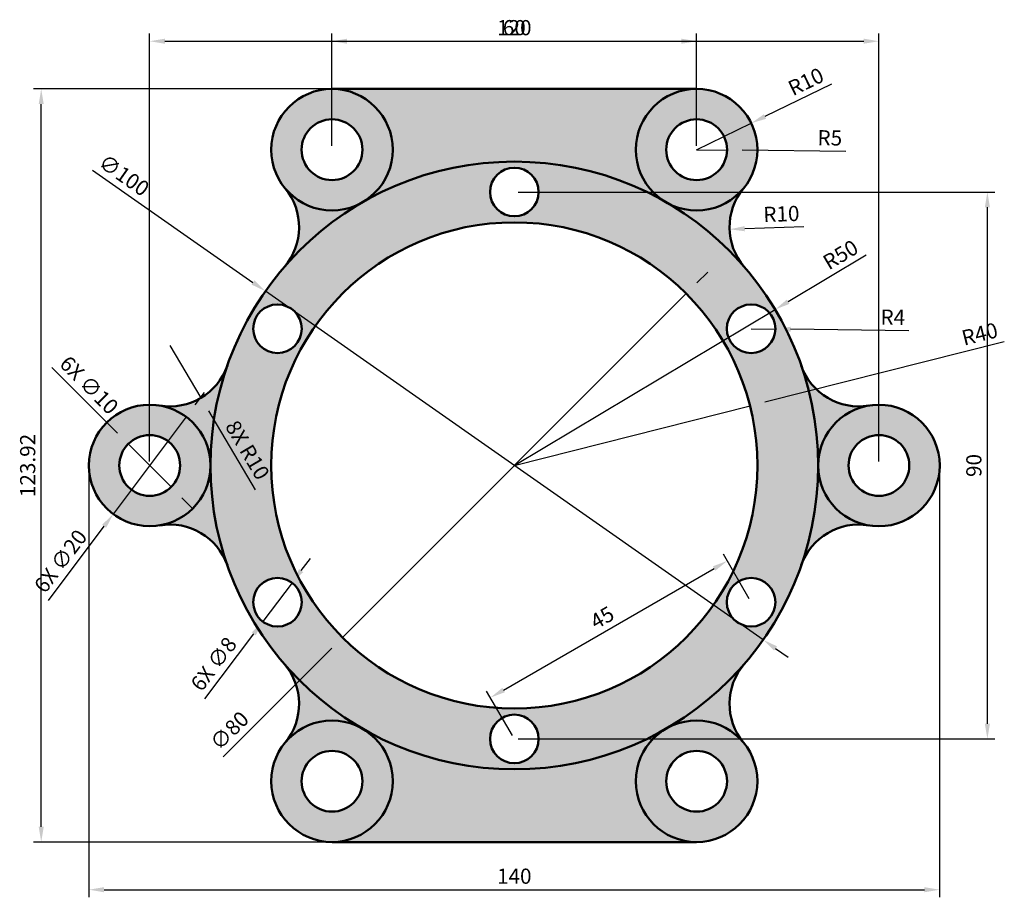
# Model space of a CAD drawing. Units: millimetres. Extents: x 1930 to 2092, y 1732 to 1877.
import ezdxf

# ---------------------------------------------------------------- set-up
doc = ezdxf.new("R2010")
doc.units = ezdxf.units.MM
for name, color, linetype, lineweight in [('M-DIMS', 2, 'Continuous', 25), ('M-HATC', 8, 'Continuous', 18), ('M-OUTL', 7, 'Continuous', 50)]:
    doc.layers.add(name, color=color, linetype=linetype, lineweight=lineweight)
doc.styles.get("Standard").update_dxf_attribs({"font": 'arial.ttf'})
doc.dimstyles.new('ISO-25', dxfattribs={"dimtxt": 2.5, "dimasz": 2.5, "dimexe": 1.25, "dimexo": 0.625, "dimtad": 1, "dimtxsty": 'Standard', "dimcen": 2.5, "dimadec": 0, "dimazin": 0, "dimtfac": 1, "dimtmove": 0, "dimatfit": 3, "dimfxl": 1, "dimarcsym": 0})

# ---------------------------------------------------------------- blocks, each defined once
blk = doc.blocks.new('*D1')
at = {"layer": 'Defpoints', "color": 0, "transparency": 16777216}
for p in [(2050.52, 1859.84), (2041.52, 1855.47)]:
    blk.add_point(p, dxfattribs=at)
at = {"layer": 'M-DIMS', "color": 0, "lineweight": -2, "transparency": 16777216}
for p, q in [((2063.73, 1866.24), (2052.77, 1860.93)), ((2041.52, 1855.47), (2050.52, 1859.84))]:
    blk.add_line(p, q, dxfattribs=at)
at = {"layer": 'M-DIMS', "color": 0, "transparency": 16777216}
blk.add_solid([(2052.59, 1861.3), (2052.95, 1860.55), (2050.52, 1859.84)], dxfattribs=at)
at = {"layer": 'M-DIMS', "color": 0, "transparency": 16777216, "insert": (2059.65, 1866.38), "char_height": 2.5, "attachment_point": 5, "rotation": 25.8634}
blk.add_mtext('R10', dxfattribs=at)
blk = doc.blocks.new('*D2')
at = {"layer": 'Defpoints', "color": 0, "transparency": 16777216}
for p in [(2041.52, 1855.47), (2046.52, 1855.41)]:
    blk.add_point(p, dxfattribs=at)
at = {"layer": 'M-DIMS', "color": 0, "lineweight": -2, "transparency": 16777216}
for p, q in [((2041.52, 1855.47), (2046.52, 1855.41)), ((2066.06, 1855.17), (2049.02, 1855.38))]:
    blk.add_line(p, q, dxfattribs=at)
at = {"layer": 'M-DIMS', "color": 0, "transparency": 16777216}
blk.add_solid([(2049.03, 1855.8), (2049.02, 1854.97), (2046.52, 1855.41)], dxfattribs=at)
at = {"layer": 'M-DIMS', "color": 0, "transparency": 16777216, "insert": (2063.44, 1857.1), "char_height": 2.5, "attachment_point": 5, "rotation": 359.2965}
blk.add_mtext('R5', dxfattribs=at)
blk = doc.blocks.new('*D3')
at = {"layer": 'Defpoints', "color": 0, "transparency": 16777216}
for p in [(2046.94, 1842.38), (2056.94, 1842.73)]:
    blk.add_point(p, dxfattribs=at)
at = {"layer": 'M-DIMS', "color": 0, "lineweight": -2, "transparency": 16777216}
blk.add_line((2059.15, 1842.8), (2049.44, 1842.47), dxfattribs=at)
at = {"layer": 'M-DIMS', "color": 0, "transparency": 16777216}
blk.add_solid([(2049.43, 1842.89), (2049.46, 1842.05), (2046.94, 1842.38)], dxfattribs=at)
at = {"layer": 'M-DIMS', "color": 0, "transparency": 16777216, "insert": (2055.48, 1844.58), "char_height": 2.5, "attachment_point": 5, "rotation": 1.9738}
blk.add_mtext('R10', dxfattribs=at)
blk = doc.blocks.new('*D4')
at = {"layer": 'Defpoints', "color": 0, "transparency": 16777216}
for p in [(2054.44, 1829.17), (2011.52, 1803.51)]:
    blk.add_point(p, dxfattribs=at)
at = {"layer": 'M-DIMS', "color": 0, "lineweight": -2, "transparency": 16777216}
for p, q in [((2069.44, 1838.14), (2056.59, 1830.45)), ((2011.52, 1803.51), (2054.44, 1829.17))]:
    blk.add_line(p, q, dxfattribs=at)
at = {"layer": 'M-DIMS', "color": 0, "transparency": 16777216}
blk.add_solid([(2056.37, 1830.81), (2056.8, 1830.1), (2054.44, 1829.17)], dxfattribs=at)
at = {"layer": 'M-DIMS', "color": 0, "transparency": 16777216, "insert": (2065.37, 1837.92), "char_height": 2.5, "attachment_point": 5, "rotation": 30.8739}
blk.add_mtext('R50', dxfattribs=at)
blk = doc.blocks.new('*D5')
at = {"layer": 'Defpoints', "color": 0, "transparency": 16777216}
for p in [(2050.5, 1826.01), (2054.5, 1825.96)]:
    blk.add_point(p, dxfattribs=at)
at = {"layer": 'M-DIMS', "color": 0, "lineweight": -2, "transparency": 16777216}
for p, q in [((2050.5, 1826.01), (2054.5, 1825.96)), ((2076.42, 1825.67), (2057, 1825.93))]:
    blk.add_line(p, q, dxfattribs=at)
at = {"layer": 'M-DIMS', "color": 0, "transparency": 16777216}
blk.add_solid([(2057, 1826.34), (2056.99, 1825.51), (2054.5, 1825.96)], dxfattribs=at)
at = {"layer": 'M-DIMS', "color": 0, "transparency": 16777216, "insert": (2073.81, 1827.58), "char_height": 2.5, "attachment_point": 5, "rotation": 359.2349}
blk.add_mtext('R4', dxfattribs=at)
blk = doc.blocks.new('*D6')
at = {"layer": 'Defpoints', "color": 0, "transparency": 16777216}
for p in [(2050.31, 1813.31), (2011.52, 1803.51)]:
    blk.add_point(p, dxfattribs=at)
at = {"layer": 'M-DIMS', "color": 0, "lineweight": -2, "transparency": 16777216}
for p, q in [((2092.16, 1823.88), (2052.73, 1813.92)), ((2011.52, 1803.51), (2050.31, 1813.31))]:
    blk.add_line(p, q, dxfattribs=at)
at = {"layer": 'M-DIMS', "color": 0, "transparency": 16777216}
blk.add_solid([(2052.63, 1814.33), (2052.83, 1813.52), (2050.31, 1813.31)], dxfattribs=at)
at = {"layer": 'M-DIMS', "color": 0, "transparency": 16777216, "insert": (2088.19, 1824.84), "char_height": 2.5, "attachment_point": 5, "rotation": 14.1779}
blk.add_mtext('R40', dxfattribs=at)
blk = doc.blocks.new('FLANGE-BOSS-D20-BORE-D10')
for radius in [10, 5]:
    blk.add_circle((10, 10), radius)
blk = doc.blocks.new('*D8')
at = {"layer": 'Defpoints', "color": 0, "transparency": 16777216}
for p in [(1941.52, 1803.51), (2081.52, 1803.51), (2081.52, 1733.7)]:
    blk.add_point(p, dxfattribs=at)
at = {"layer": 'M-DIMS', "color": 0, "lineweight": -2, "transparency": 16777216}
for p, q in [((1941.52, 1802.89), (1941.52, 1732.45)), ((2081.52, 1802.89), (2081.52, 1732.45)), ((1944.02, 1733.7), (2079.02, 1733.7))]:
    blk.add_line(p, q, dxfattribs=at)
at = {"layer": 'M-DIMS', "color": 0, "transparency": 16777216}
for points in [[(1944.02, 1734.12), (1944.02, 1733.28), (1941.52, 1733.7)], [(2079.02, 1734.12), (2079.02, 1733.28), (2081.52, 1733.7)]]:
    blk.add_solid(points, dxfattribs=at)
at = {"layer": 'M-DIMS', "color": 0, "transparency": 16777216, "insert": (2011.52, 1735.6), "char_height": 2.5, "attachment_point": 5}
blk.add_mtext('140', dxfattribs=at)
blk = doc.blocks.new('*D9')
at = {"layer": 'Defpoints', "color": 0, "transparency": 16777216}
for p in [(1933.67, 1865.47), (1981.52, 1865.47), (1981.52, 1741.55)]:
    blk.add_point(p, dxfattribs=at)
at = {"layer": 'M-DIMS', "color": 0, "lineweight": -2, "transparency": 16777216}
for p, q in [((1980.9, 1865.47), (1932.42, 1865.47)), ((1933.67, 1744.05), (1933.67, 1862.97)), ((1980.9, 1741.55), (1932.42, 1741.55))]:
    blk.add_line(p, q, dxfattribs=at)
at = {"layer": 'M-DIMS', "color": 0, "transparency": 16777216}
for points in [[(1933.26, 1862.97), (1934.09, 1862.97), (1933.67, 1865.47)], [(1933.26, 1744.05), (1934.09, 1744.05), (1933.67, 1741.55)]]:
    blk.add_solid(points, dxfattribs=at)
at = {"layer": 'M-DIMS', "color": 0, "transparency": 16777216, "insert": (1931.77, 1803.51), "char_height": 2.5, "attachment_point": 5, "rotation": 90}
blk.add_mtext('123.92', dxfattribs=at)
blk = doc.blocks.new('*D10')
at = {"layer": 'Defpoints', "color": 0, "transparency": 16777216}
for p in [(2071.52, 1873.32), (1951.52, 1803.51), (2071.52, 1803.51)]:
    blk.add_point(p, dxfattribs=at)
at = {"layer": 'M-DIMS', "color": 0, "lineweight": -2, "transparency": 16777216}
for p, q in [((1951.52, 1804.14), (1951.52, 1874.57)), ((1954.02, 1873.32), (2069.02, 1873.32)), ((2071.52, 1804.14), (2071.52, 1874.57))]:
    blk.add_line(p, q, dxfattribs=at)
at = {"layer": 'M-DIMS', "color": 0, "transparency": 16777216}
for points in [[(1954.02, 1873.74), (1954.02, 1872.91), (1951.52, 1873.32)], [(2069.02, 1873.74), (2069.02, 1872.91), (2071.52, 1873.32)]]:
    blk.add_solid(points, dxfattribs=at)
at = {"layer": 'M-DIMS', "color": 0, "transparency": 16777216, "insert": (2011.52, 1875.23), "char_height": 2.5, "attachment_point": 5}
blk.add_mtext('120', dxfattribs=at)
blk = doc.blocks.new('*D11')
at = {"layer": 'Defpoints', "color": 0, "transparency": 16777216}
for p in [(2011.52, 1848.51), (2089.37, 1848.51), (2011.52, 1758.51)]:
    blk.add_point(p, dxfattribs=at)
at = {"layer": 'M-DIMS', "color": 0, "lineweight": -2, "transparency": 16777216}
for p, q in [((2012.15, 1848.51), (2090.62, 1848.51)), ((2089.37, 1761.01), (2089.37, 1846.01)), ((2012.15, 1758.51), (2090.62, 1758.51))]:
    blk.add_line(p, q, dxfattribs=at)
at = {"layer": 'M-DIMS', "color": 0, "transparency": 16777216}
for points in [[(2088.96, 1846.01), (2089.79, 1846.01), (2089.37, 1848.51)], [(2088.96, 1761.01), (2089.79, 1761.01), (2089.37, 1758.51)]]:
    blk.add_solid(points, dxfattribs=at)
at = {"layer": 'M-DIMS', "color": 0, "transparency": 16777216, "insert": (2087.47, 1803.51), "char_height": 2.5, "attachment_point": 5, "rotation": 90}
blk.add_mtext('90', dxfattribs=at)
blk = doc.blocks.new('*D12')
at = {"layer": 'Defpoints', "color": 0, "transparency": 16777216}
for p in [(2041.52, 1873.32), (1981.52, 1855.47), (2041.52, 1855.47)]:
    blk.add_point(p, dxfattribs=at)
at = {"layer": 'M-DIMS', "color": 0, "lineweight": -2, "transparency": 16777216}
for p, q in [((1981.52, 1856.1), (1981.52, 1874.57)), ((1984.02, 1873.32), (2039.02, 1873.32)), ((2041.52, 1856.1), (2041.52, 1874.57))]:
    blk.add_line(p, q, dxfattribs=at)
at = {"layer": 'M-DIMS', "color": 0, "transparency": 16777216}
for points in [[(1984.02, 1873.74), (1984.02, 1872.91), (1981.52, 1873.32)], [(2039.02, 1873.74), (2039.02, 1872.91), (2041.52, 1873.32)]]:
    blk.add_solid(points, dxfattribs=at)
at = {"layer": 'M-DIMS', "color": 0, "transparency": 16777216, "insert": (2011.52, 1875.23), "char_height": 2.5, "attachment_point": 5}
blk.add_mtext('60', dxfattribs=at)
blk = doc.blocks.new('*D13')
at = {"layer": 'Defpoints', "color": 0, "transparency": 16777216}
for p in [(2046.57, 1787.81), (2050.5, 1781.01), (2011.52, 1758.51)]:
    blk.add_point(p, dxfattribs=at)
at = {"layer": 'M-DIMS', "color": 0, "lineweight": -2, "transparency": 16777216}
for p, q in [((2050.18, 1781.55), (2045.95, 1788.89)), ((2009.76, 1766.56), (2044.41, 1786.56)), ((2011.21, 1759.05), (2006.97, 1766.39))]:
    blk.add_line(p, q, dxfattribs=at)
at = {"layer": 'M-DIMS', "color": 0, "transparency": 16777216}
for points in [[(2044.2, 1786.92), (2044.61, 1786.2), (2046.57, 1787.81)], [(2009.56, 1766.92), (2009.97, 1766.2), (2007.6, 1765.31)]]:
    blk.add_solid(points, dxfattribs=at)
at = {"layer": 'M-DIMS', "color": 0, "transparency": 16777216, "insert": (2026.14, 1778.2), "char_height": 2.5, "attachment_point": 5, "rotation": 30}
blk.add_mtext('45', dxfattribs=at)
blk = doc.blocks.new('*D14')
at = {"layer": 'Defpoints', "color": 0, "transparency": 16777216}
for p in [(1970.57, 1832.19), (2052.48, 1774.83)]:
    blk.add_point(p, dxfattribs=at)
at = {"layer": 'M-DIMS', "color": 0, "lineweight": -2, "transparency": 16777216}
for p, q in [((1942.11, 1852.12), (1968.52, 1833.62)), ((2052.48, 1774.83), (1970.57, 1832.19)), ((2054.53, 1773.4), (2056.58, 1771.97))]:
    blk.add_line(p, q, dxfattribs=at)
at = {"layer": 'M-DIMS', "color": 0, "transparency": 16777216}
for points in [[(1968.76, 1833.97), (1968.28, 1833.28), (1970.57, 1832.19)], [(2054.77, 1773.74), (2054.29, 1773.06), (2052.48, 1774.83)]]:
    blk.add_solid(points, dxfattribs=at)
at = {"layer": 'M-DIMS', "color": 0, "transparency": 16777216, "insert": (1947.12, 1851.01), "char_height": 2.5, "attachment_point": 5, "rotation": 325.0002}
blk.add_mtext('∅100', dxfattribs=at)
blk = doc.blocks.new('*D15')
at = {"layer": 'Defpoints', "color": 0, "transparency": 16777216}
for p in [(2039.81, 1831.8), (1983.24, 1775.23)]:
    blk.add_point(p, dxfattribs=at)
at = {"layer": 'M-DIMS', "color": 0, "lineweight": -2, "transparency": 16777216}
for p, q in [((2041.58, 1833.56), (2043.35, 1835.33)), ((2039.81, 1831.8), (1983.24, 1775.23)), ((1963.6, 1755.59), (1981.47, 1773.46))]:
    blk.add_line(p, q, dxfattribs=at)
at = {"layer": 'M-DIMS', "color": 0, "transparency": 16777216}
for points in [[(2041.28, 1833.86), (2041.87, 1833.27), (2039.81, 1831.8)], [(1981.18, 1773.76), (1981.77, 1773.17), (1983.24, 1775.23)]]:
    blk.add_solid(points, dxfattribs=at)
at = {"layer": 'M-DIMS', "color": 0, "transparency": 16777216, "insert": (1964.87, 1759.65), "char_height": 2.5, "attachment_point": 5, "rotation": 44.9978}
blk.add_mtext('∅80', dxfattribs=at)
blk = doc.blocks.new('*D16')
at = {"layer": 'Defpoints', "color": 0, "transparency": 16777216}
for p in [(1954.86, 1823.23), (1959.95, 1814.63)]:
    blk.add_point(p, dxfattribs=at)
at = {"layer": 'M-DIMS', "color": 0, "lineweight": -2, "transparency": 16777216}
for p, q in [((1954.86, 1823.23), (1959.95, 1814.63)), ((1968.91, 1799.49), (1961.23, 1812.48))]:
    blk.add_line(p, q, dxfattribs=at)
at = {"layer": 'M-DIMS', "color": 0, "transparency": 16777216}
blk.add_solid([(1961.58, 1812.69), (1960.87, 1812.26), (1959.95, 1814.63)], dxfattribs=at)
at = {"layer": 'M-DIMS', "color": 0, "transparency": 16777216, "insert": (1967.34, 1805.88), "char_height": 2.5, "attachment_point": 5, "rotation": 300.6218}
blk.add_mtext('8X R10', dxfattribs=at)
blk = doc.blocks.new('*D17')
at = {"layer": 'Defpoints', "color": 0, "transparency": 16777216}
for p in [(1957.52, 1811.51), (1945.53, 1795.51)]:
    blk.add_point(p, dxfattribs=at)
at = {"layer": 'M-DIMS', "color": 0, "lineweight": -2, "transparency": 16777216}
for p, q in [((1959.02, 1813.51), (1960.52, 1815.51)), ((1957.52, 1811.51), (1945.53, 1795.51)), ((1934.85, 1781.28), (1944.03, 1793.51))]:
    blk.add_line(p, q, dxfattribs=at)
at = {"layer": 'M-DIMS', "color": 0, "transparency": 16777216}
for points in [[(1958.69, 1813.76), (1959.36, 1813.26), (1957.52, 1811.51)], [(1943.69, 1793.76), (1944.36, 1793.26), (1945.53, 1795.51)]]:
    blk.add_solid(points, dxfattribs=at)
at = {"layer": 'M-DIMS', "color": 0, "transparency": 16777216, "insert": (1937.11, 1787.58), "char_height": 2.5, "attachment_point": 5, "rotation": 53.1332}
blk.add_mtext('6X ∅20', dxfattribs=at)
blk = doc.blocks.new('*D18')
at = {"layer": 'Defpoints', "color": 0, "transparency": 16777216}
for p in [(1947.99, 1807.05), (1955.06, 1799.98)]:
    blk.add_point(p, dxfattribs=at)
at = {"layer": 'M-DIMS', "color": 0, "lineweight": -2, "transparency": 16777216}
for p, q in [((1935.41, 1819.64), (1946.22, 1808.82)), ((1955.06, 1799.98), (1947.99, 1807.05)), ((1956.83, 1798.21), (1958.59, 1796.44))]:
    blk.add_line(p, q, dxfattribs=at)
at = {"layer": 'M-DIMS', "color": 0, "transparency": 16777216}
for points in [[(1946.52, 1809.11), (1945.93, 1808.52), (1947.99, 1807.05)], [(1957.12, 1798.5), (1956.53, 1797.91), (1955.06, 1799.98)]]:
    blk.add_solid(points, dxfattribs=at)
at = {"layer": 'M-DIMS', "color": 0, "transparency": 16777216, "insert": (1941.33, 1816.51), "char_height": 2.5, "attachment_point": 5, "rotation": 314.9761}
blk.add_mtext('6X ∅10', dxfattribs=at)
blk = doc.blocks.new('*D19')
at = {"layer": 'Defpoints', "color": 0, "transparency": 16777216}
for p in [(1974.96, 1784.21), (1970.15, 1777.81)]:
    blk.add_point(p, dxfattribs=at)
at = {"layer": 'M-DIMS', "color": 0, "lineweight": -2, "transparency": 16777216}
for p, q in [((1976.46, 1786.21), (1977.96, 1788.21)), ((1974.96, 1784.21), (1970.15, 1777.81)), ((1960.62, 1765.13), (1968.65, 1775.81))]:
    blk.add_line(p, q, dxfattribs=at)
at = {"layer": 'M-DIMS', "color": 0, "transparency": 16777216}
for points in [[(1976.12, 1786.46), (1976.79, 1785.96), (1974.96, 1784.21)], [(1968.32, 1776.07), (1968.98, 1775.56), (1970.15, 1777.81)]]:
    blk.add_solid(points, dxfattribs=at)
at = {"layer": 'M-DIMS', "color": 0, "transparency": 16777216, "insert": (1962.31, 1770.66), "char_height": 2.5, "attachment_point": 5, "rotation": 53.0937}
blk.add_mtext('6X ∅8', dxfattribs=at)

msp = doc.modelspace()

# ---------------------------------------------------------------- hatches: boundary and pattern name
at = {"layer": 'M-HATC'}
h = msp.add_hatch(color=256, dxfattribs=at)
h.dxf.hatch_style = 1
h.set_gradient(color1=(255, 0, 0), color2=(255, 255, 0), tint=1, name='CYLINDER')
h.paths.add_polyline_path([(1991.525, 1855.474, 1), (1971.525, 1855.474, 1)])
h.paths.add_polyline_path([(1976.525, 1855.474, -1), (1986.525, 1855.474, -1)], flags=16)
h.paths.add_polyline_path([(2051.525, 1855.474, 1), (2031.525, 1855.474, 1)])
h.paths.add_polyline_path([(2036.525, 1855.474, -1), (2046.525, 1855.474, -1)], flags=16)
h.paths.add_polyline_path([(1941.525, 1803.512, 1), (1961.525, 1803.512, 1)])
h.paths.add_polyline_path([(1956.525, 1803.512, -1), (1946.525, 1803.512, -1)], flags=16)
h.paths.add_polyline_path([(2061.525, 1803.512, 1), (2081.525, 1803.512, 1)])
h.paths.add_polyline_path([(2076.525, 1803.512, -1), (2066.525, 1803.512, -1)], flags=16)
h.paths.add_polyline_path([(2031.525, 1751.551, 1), (2051.525, 1751.551, 1)])
h.paths.add_polyline_path([(2046.525, 1751.551, -1), (2036.525, 1751.551, -1)], flags=16)
h.paths.add_polyline_path([(1971.525, 1751.551, 1), (1991.525, 1751.551, 1)])
h.paths.add_polyline_path([(1976.525, 1751.551, -1), (1986.525, 1751.551, -1)], flags=16)
h = msp.add_hatch(color=256, dxfattribs=at)
h.dxf.hatch_style = 1
h.set_gradient(color1=(0, 0, 255), color2=(255, 255, 0), tint=1, name='CYLINDER')
h.paths.add_polyline_path([(1961.525, 1803.512, 1), (2061.525, 1803.512, 1)])
h.paths.add_polyline_path([(2051.525, 1803.512, -1), (1971.525, 1803.512, -1)], flags=16)
h.paths.add_polyline_path([(2007.525, 1848.512, -1), (2015.525, 1848.512, -1)], flags=16)
h.paths.add_polyline_path([(2054.496, 1826.012, -1), (2046.496, 1826.012, -1)], flags=16)
h.paths.add_polyline_path([(1976.553, 1826.012, -1), (1968.553, 1826.012, -1)], flags=16)
h.paths.add_polyline_path([(2054.496, 1781.012, -1), (2046.496, 1781.012, -1)], flags=16)
h.paths.add_polyline_path([(1976.553, 1781.012, -1), (1968.553, 1781.012, -1)], flags=16)
h.paths.add_polyline_path([(2015.525, 1758.512, -1), (2007.525, 1758.512, -1)], flags=16)
h.paths.add_polyline_path([(2041.525, 1865.474), (1981.525, 1865.474, -0.4142136), (1991.525, 1855.474, -0.2679492), (1986.525, 1846.814, -0.2679492), (2036.525, 1846.814, -0.2679492), (2031.525, 1855.474, -0.4142136)])
h.paths.add_polyline_path([(2031.525, 1751.551, -0.2679492), (2036.525, 1760.211, -0.2679492), (1986.525, 1760.211, -0.2679492), (1991.525, 1751.551, -0.4142136), (1981.525, 1741.551), (2041.525, 1741.551, -0.4142136)])
h.paths.add_polyline_path([(1986.525, 1846.814, -0.3659774), (1973.819, 1849.101, -0.3659774), (1973.682, 1836.191, -0.0839202)], flags=17)
h.paths.add_polyline_path([(1964.302, 1819.946, -0.3659774), (1953.191, 1813.373, -0.3659774), (1961.525, 1803.512, -0.0839202)])
h.paths.add_polyline_path([(1961.525, 1803.512, -0.3659774), (1953.191, 1793.652, -0.3659774), (1964.302, 1787.079, -0.0839202)])
h.paths.add_polyline_path([(2049.23, 1849.101, -0.3659774), (2036.525, 1846.814, -0.0839202), (2049.368, 1836.191, -0.3659774)], flags=17)
h.paths.add_polyline_path([(2069.858, 1813.373, -0.3659774), (2058.747, 1819.946, -0.0839202), (2061.525, 1803.512, -0.3659774)])
h.paths.add_polyline_path([(2061.525, 1803.512, -0.0839202), (2058.747, 1787.079, -0.3659774), (2069.858, 1793.652, -0.3659774)])
h.paths.add_polyline_path([(1973.682, 1770.834, -0.3659774), (1973.819, 1757.924, -0.3659774), (1986.525, 1760.211, -0.0839202)], flags=17)
h.paths.add_polyline_path([(2049.368, 1770.834, -0.0839202), (2036.525, 1760.211, -0.3659774), (2049.23, 1757.924, -0.3659774)], flags=17)

# ---------------------------------------------------------------- linework, layer by layer
at = {"layer": 'M-OUTL'}
for p, q in [((1981.525, 1865.474), (2041.525, 1865.474)), ((1981.525, 1741.551), (2041.525, 1741.551))]:
    msp.add_line(p, q, dxfattribs=at)
for centre, radius in [((2011.525, 1803.512), 50), ((2011.525, 1848.512), 4), ((2011.525, 1803.512), 40), ((1972.553, 1826.012), 4), ((2050.496, 1826.012), 4), ((1972.553, 1781.012), 4), ((2050.496, 1781.012), 4), ((2011.525, 1758.512), 4)]:
    msp.add_circle(centre, radius, dxfattribs=at)
for centre, start, end in [((1966.113, 1842.727), 319.18814, 39.59407), ((2056.936, 1842.727), 140.40593, 220.81186), ((1954.858, 1823.233), 260.40593, 340.81186), ((2068.191, 1823.233), 199.18814, 279.59407), ((1954.858, 1783.792), 19.18814, 99.59407), ((2068.191, 1783.792), 80.40593, 160.81186), ((1966.113, 1764.298), 320.40593, 40.81186), ((2056.936, 1764.298), 139.18814, 219.59407)]:
    msp.add_arc(centre, 10, start, end, dxfattribs=at)

# ---------------------------------------------------------------- block references
for p in [(1971.525, 1845.474), (2031.525, 1845.474), (2061.525, 1793.512), (1971.525, 1741.551)]:
    msp.add_blockref('FLANGE-BOSS-D20-BORE-D10', p, dxfattribs=at)
at = {"layer": 'M-OUTL', "rotation": 90}
for p in [(1961.525, 1793.513), (2051.525, 1741.551)]:
    msp.add_blockref('FLANGE-BOSS-D20-BORE-D10', p, dxfattribs=at)

# ---------------------------------------------------------------- dimensions: what is measured, and where the dimension line sits
at = {"layer": 'M-DIMS'}
for base, p1, p2, picture, middle in [((2071.525, 1873.324), (1951.525, 1803.512), (2071.525, 1803.512), '*D10', (2011.525, 1875.225)), ((2041.525, 1873.324), (1981.525, 1855.474), (2041.525, 1855.474), '*D12', (2011.525, 1875.225)), ((2081.525, 1733.701), (1941.525, 1803.512), (2081.525, 1803.512), '*D8', (2011.525, 1735.602))]:
    dim = msp.add_linear_dim(base=base, p1=p1, p2=p2, dimstyle='ISO-25', override={"dimdec": 0, "dimlfac": 1, "dimrnd": 0, "dimzin": 0, "dimdsep": 46, "dimlunit": 2}, dxfattribs=at)
    dim.commit()
    dim.dimension.update_dxf_attribs({"geometry": picture, "text_midpoint": middle})
for center, mpoint, picture, middle in [((2041.525, 1855.474), (2050.523, 1859.836), '*D1', (2060.482, 1864.664)), ((2041.525, 1855.474), (2046.524, 1855.413), '*D2', (2063.413, 1855.205)), ((2056.936, 1842.727), (2046.942, 1842.383), '*D3', (2055.545, 1842.679)), ((2011.525, 1803.512), (2054.44, 1829.17), '*D4', (2066.343, 1836.287)), ((2050.496, 1826.012), (2054.495, 1825.959), '*D5', (2073.782, 1825.701)), ((2011.525, 1803.512), (2050.306, 1813.31), '*D6', (2088.659, 1822.999))]:
    dim = msp.add_radius_dim(center=center, mpoint=mpoint, dimstyle='ISO-25', override={"dimclrd": 0, "dimclre": 0, "dimclrt": 0}, dxfattribs=at)
    dim.commit()
    dim.dimension.update_dxf_attribs({"geometry": picture, "text_midpoint": middle, "dimtype": 164})
for base, p1, p2, angle, override, picture, middle in [((1933.675, 1865.474), (1981.525, 1741.551), (1981.525, 1865.474), 90, {"dimdec": 2, "dimlfac": 1, "dimrnd": 0, "dimzin": 0, "dimdsep": 46, "dimlunit": 2}, '*D9', (1931.772, 1803.512)), ((2089.375, 1848.512), (2011.525, 1758.512), (2011.525, 1848.512), 90, {"dimdec": 0, "dimlfac": 1, "dimrnd": 0, "dimzin": 0, "dimdsep": 46, "dimlunit": 2}, '*D11', (2087.473, 1803.512)), ((2046.571, 1787.811), (2011.525, 1758.512), (2050.496, 1781.012), 30, {"dimdec": 0, "dimlfac": 1, "dimrnd": 0, "dimzin": 0, "dimdsep": 46, "dimlunit": 2}, '*D13', (2026.137, 1778.203))]:
    dim = msp.add_linear_dim(base=base, p1=p1, p2=p2, angle=angle, dimstyle='ISO-25', override=override, dxfattribs=at)
    dim.commit()
    dim.dimension.update_dxf_attribs({"geometry": picture, "text_midpoint": middle})
for p1, p2, picture, middle in [((2052.482, 1774.834), (1970.567, 1832.191), '*D14', (1945.992, 1849.398)), ((2039.81, 1831.796), (1983.239, 1775.229), '*D15', (1966.268, 1758.259))]:
    dim = msp.add_diameter_dim_2p(p1=p1, p2=p2, dimstyle='ISO-25', override={"dimdec": 0, "dimlfac": 1, "dimrnd": 0, "dimzin": 0, "dimdsep": 46, "dimlunit": 2}, dxfattribs=at)
    dim.commit()
    dim.dimension.update_dxf_attribs({"geometry": picture, "text_midpoint": middle, "dimtype": 163})
dim = msp.add_radius_dim(center=(1954.858, 1823.233), mpoint=(1959.952, 1814.627), text='8X <>', dimstyle='ISO-25', override={"dimdec": 0, "dimlfac": 1, "dimrnd": 0, "dimzin": 0, "dimdsep": 46, "dimlunit": 2}, dxfattribs=at)
dim.commit()
dim.dimension.update_dxf_attribs({"geometry": '*D16', "text_midpoint": (1967.341, 1805.876)})
for p1, p2, picture, middle in [((1955.059, 1799.975), (1947.991, 1807.049), '*D18', (1939.935, 1815.112)), ((1957.524, 1811.513), (1945.525, 1795.512), '*D17', (1938.687, 1786.394))]:
    dim = msp.add_diameter_dim_2p(p1=p1, p2=p2, text='6X <>', dimstyle='ISO-25', override={"dimdec": 0, "dimlfac": 1, "dimrnd": 0, "dimzin": 0, "dimdsep": 46, "dimlunit": 2}, dxfattribs=at)
    dim.commit()
    dim.dimension.update_dxf_attribs({"geometry": picture, "text_midpoint": middle, "dimtype": 163})
dim = msp.add_diameter_dim_2p(p1=(1974.956, 1784.211), p2=(1970.151, 1777.814), text='6X <>', dimstyle='ISO-25', override={"dimdec": 0, "dimlfac": 1, "dimrnd": 0, "dimzin": 0, "dimdsep": 46, "dimlunit": 2}, dxfattribs=at)
dim.commit()
dim.dimension.update_dxf_attribs({"geometry": '*D19', "text_midpoint": (1963.886, 1769.471)})

doc.saveas('drawing.dxf')
